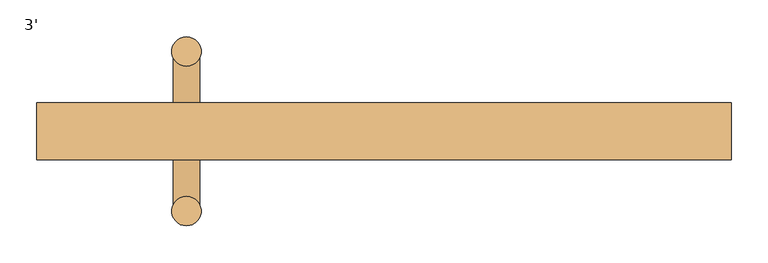
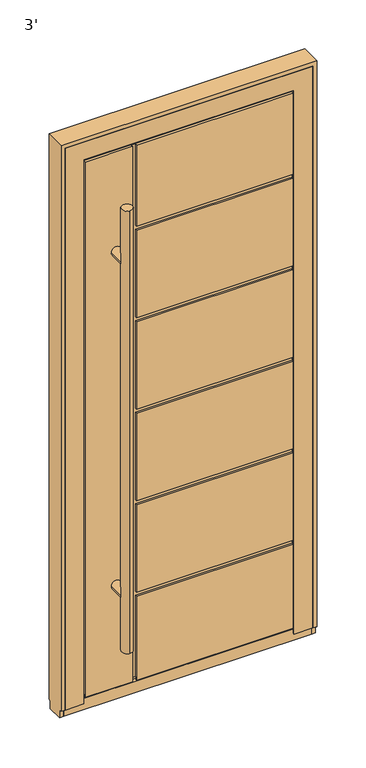
"""IFC4 building model written with IfcOpenShell, lengths in millimetres: door geometry, 3'."""

from ifc_helpers import new_model, si_unit, point, frame, frame_2d, origin, place, context, project, spatial, circle_curve, trimmed, segment, composite_curve, outline, extrude, faceted_brep, source, transform, mapped, element, save


def door_3_5c4206ef(model_context):
    return source(origin(), model_context, "Body", "SolidModel", [
        extrude(outline(composite_curve([segment(trimmed(circle_curve(frame_2d((-268.65, -90.8003001)), 20.0), [point((-268.65, -70.8003001))], [point((-268.65, -110.8003001))], False, "CARTESIAN"), True, "CONTINUOUS"), segment(trimmed(circle_curve(frame_2d((-268.65, -90.8003001)), 20.0), [point((-268.65, -110.8003001))], [point((-268.65, -70.8003001))], False, "CARTESIAN"), True, "CONTINUOUS")], self_intersect=False)), frame((0.0, 0.0, 210.0000003), z_axis=(0.0, 0.0, 1.0), x_axis=(1.0, 0.0, 0.0)), (0.0, 0.0, 1.0), 1724.5),
        extrude(outline(composite_curve([segment(trimmed(circle_curve(frame_2d((-268.65, 126.2003001)), 20.0), [point((-268.65, 146.2003001))], [point((-268.65, 106.2003001))], False, "CARTESIAN"), True, "CONTINUOUS"), segment(trimmed(circle_curve(frame_2d((-268.65, 126.2003001)), 20.0), [point((-268.65, 106.2003001))], [point((-268.65, 146.2003001))], False, "CARTESIAN"), True, "CONTINUOUS")], self_intersect=False)), frame((0.0, 0.0, 210.0000003), z_axis=(0.0, 0.0, 1.0), x_axis=(1.0, 0.0, 0.0)), (0.0, 0.0, 1.0), 1724.5),
        extrude(outline(composite_curve([segment(trimmed(circle_curve(frame_2d((422.2500003, -268.65)), 18.0), [point((422.2500003, -286.65))], [point((422.2500003, -250.65))], False, "CARTESIAN"), True, "CONTINUOUS"), segment(trimmed(circle_curve(frame_2d((422.2500003, -268.65)), 18.0), [point((422.2500003, -250.65))], [point((422.2500003, -286.65))], False, "CARTESIAN"), True, "CONTINUOUS")], self_intersect=False)), frame((0.0, -90.8, 0.0), z_axis=(0.0, 1.0, 0.0), x_axis=(0.0, 0.0, 1.0)), (0.0, 0.0, 1.0), 217.0),
        extrude(outline(composite_curve([segment(trimmed(circle_curve(frame_2d((1722.2500003, -268.65)), 18.0), [point((1722.2500003, -286.65))], [point((1722.2500003, -250.65))], False, "CARTESIAN"), True, "CONTINUOUS"), segment(trimmed(circle_curve(frame_2d((1722.2500003, -268.65)), 18.0), [point((1722.2500003, -250.65))], [point((1722.2500003, -286.65))], False, "CARTESIAN"), True, "CONTINUOUS")], self_intersect=False)), frame((0.0, -90.8, 0.0), z_axis=(0.0, 1.0, 0.0), x_axis=(0.0, 0.0, 1.0)), (0.0, 0.0, 1.0), 217.0),
        faceted_brep([(-193.65, -13.8, 366.5833337), (-193.65, -13.8, 708.166667), (383.65, -13.8, 708.166667), (383.65, -13.8, 723.166667), (-193.65, -13.8, 723.166667), (-193.65, -13.8, 1064.7500004), (383.65, -13.8, 1064.7500004), (383.65, -13.8, 1079.7500004), (-193.65, -13.8, 1079.7500004), (-193.65, -13.8, 1421.3333337), (383.65, -13.8, 1421.3333337), (383.65, -13.8, 1436.3333337), (-193.65, -13.8, 1436.3333337), (-193.65, -13.8, 1777.916667), (383.65, -13.8, 1777.916667), (383.65, -13.8, 1792.916667), (-193.65, -13.8, 1792.916667), (-193.65, -13.8, 2109.5000003), (-208.65, -13.8, 2109.5000003), (-208.65, -13.8, 35.0), (-193.65, -13.8, 35.0), (-193.65, -13.8, 351.5833337), (383.65, -13.8, 351.5833337), (383.65, -13.8, 366.5833337), (-193.65, -20.8, 366.5833337), (-193.65, -20.8, 708.166667), (383.65, -20.8, 708.166667), (383.65, -11.7997698, 2109.5000003), (383.65, -20.8, 2109.5000003), (383.65, -20.8, 1792.916667), (383.65, -20.8, 1777.916667), (383.65, -20.8, 1436.3333337), (383.65, -20.8, 1421.3333337), (383.65, -20.8, 1079.7500004), (383.65, -20.8, 1064.7500004), (383.65, -20.8, 723.166667), (383.65, -20.8, 366.5833337), (383.65, -20.8, 351.5833337), (383.65, -20.8, 24.0), (383.65, -18.8020472, 24.0), (383.65, -18.8020472, 35.0), (383.65, -11.7997698, 35.0), (-193.65, -20.8, 723.166667), (-193.65, -20.8, 1064.7500004), (-193.65, -20.8, 1079.7500004), (-193.65, -20.8, 1421.3333337), (-208.65, -20.8, 2109.5000003), (-208.65, -20.8, 24.0), (-208.65, -18.8020472, 24.0), (-208.65, -18.8020472, 35.0), (-193.65, -18.8020472, 35.0), (-383.65, -18.8020472, 35.0), (-383.65, -11.7997698, 35.0), (-193.65, -20.8, 351.5833337), (-193.65, -18.8020472, 24.0), (-193.65, -20.8, 24.0), (-383.65, -18.8020472, 24.0), (-383.65, -20.8, 24.0), (-383.65, -20.8, 2109.5000003), (-193.65, -20.8, 1777.916667), (-193.65, -20.8, 1436.3333337), (-193.65, -20.8, 2109.5000003), (-193.65, -20.8, 1792.916667), (408.65, 56.2, 10.0000003), (408.65, 53.2, 10.0000003), (-193.65, 53.2, 10.0000003), (-193.65, 56.2, 10.0000003), (-408.65, 53.2, 10.0000003), (-408.65, 56.2, 10.0000003), (-208.65, 56.2, 10.0000003), (-208.65, 53.2, 10.0000003), (408.65, 56.2, 351.5833337), (408.65, 53.2, 351.5833337), (408.65, 56.2, 366.5833337), (408.65, 56.2, 708.166667), (408.65, 53.2, 708.166667), (408.65, 53.2, 366.5833337), (408.65, 56.2, 1079.7500004), (408.65, 56.2, 1421.3333337), (408.65, 53.2, 1421.3333337), (408.65, 53.2, 1079.7500004), (408.65, 56.2, 723.166667), (408.65, 56.2, 1064.7500004), (408.65, 53.2, 1064.7500004), (408.65, 53.2, 723.166667), (408.65, 56.2, 1436.3333337), (408.65, 56.2, 1777.916667), (408.65, 53.2, 1777.916667), (408.65, 53.2, 1436.3333337), (408.65, 56.2, 2134.5000003), (408.65, 53.2, 2134.5000003), (408.65, 53.2, 1792.916667), (408.65, 56.2, 1792.916667), (393.15, 53.2, 351.5833337), (393.15, 53.2, 25.5), (-193.65, 53.2, 25.5), (393.15, 53.2, 708.166667), (393.15, 53.2, 366.5833337), (393.15, 53.2, 1421.3333337), (393.15, 53.2, 1079.7500004), (393.15, 53.2, 1064.7500004), (393.15, 53.2, 723.166667), (393.15, 53.2, 1777.916667), (393.15, 53.2, 1436.3333337), (-193.65, 53.2, 2134.5000003), (-193.65, 53.2, 2119.0000003), (393.15, 53.2, 2119.0000003), (393.15, 53.2, 1792.916667), (-393.15, 53.2, 25.5), (-393.15, 53.2, 2119.0000003), (-208.65, 53.2, 2119.0000003), (-208.65, 53.2, 2134.5000003), (-408.65, 53.2, 2134.5000003), (-208.65, 53.2, 25.5), (-193.65, 49.2, 351.5833337), (-193.65, 56.2, 351.5833337), (-193.65, 49.2, 25.5), (-193.65, 56.2, 366.5833337), (-193.65, 56.2, 708.166667), (-193.65, 56.2, 1079.7500004), (-193.65, 56.2, 1421.3333337), (-193.65, 56.2, 723.166667), (-193.65, 56.2, 1064.7500004), (-193.65, 56.2, 1436.3333337), (-193.65, 56.2, 1777.916667), (-193.65, 56.2, 1792.916667), (-193.65, 56.2, 2134.5000003), (-408.65, 56.2, 2134.5000003), (-208.65, 56.2, 2134.5000003), (-208.65, 49.2, 2119.0000003), (-208.65, 49.2, 25.5), (-383.65, -11.7997698, 2109.5000003), (393.15, -11.7997698, 2119.0000003), (-393.15, -11.7997698, 2119.0000003), (-393.15, -11.7997698, 25.5), (393.15, -11.7997698, 25.5), (393.15, 49.2, 351.5833337), (393.15, 49.2, 366.5833337), (393.15, 49.2, 708.166667), (393.15, 49.2, 723.166667), (393.15, 49.2, 1064.7500004), (393.15, 49.2, 1079.7500004), (393.15, 49.2, 1421.3333337), (393.15, 49.2, 1436.3333337), (393.15, 49.2, 1777.916667), (393.15, 49.2, 1792.916667), (-193.65, 49.2, 1777.916667), (-193.65, 49.2, 1436.3333337), (-193.65, 49.2, 1421.3333337), (-193.65, 49.2, 1079.7500004), (-193.65, 49.2, 1064.7500004), (-193.65, 49.2, 723.166667), (-193.65, 49.2, 708.166667), (-193.65, 49.2, 366.5833337), (-193.65, 49.2, 2119.0000003), (-193.65, 49.2, 1792.916667)], [[[0, 1, 2, 3, 4, 5, 6, 7, 8, 9, 10, 11, 12, 13, 14, 15, 16, 17, 18, 19, 20, 21, 22, 23]], [[1, 0, 24, 25]], [[1, 25, 26, 2]], [[27, 28, 29, 15, 14, 30, 31, 11, 10, 32, 33, 7, 6, 34, 35, 3, 2, 26, 36, 23, 22, 37, 38, 39, 40, 41]], [[42, 4, 3, 35]], [[5, 4, 42, 43]], [[5, 43, 34, 6]], [[44, 8, 7, 33]], [[9, 8, 44, 45]], [[19, 18, 46, 47, 48, 49]], [[41, 40, 50, 20, 19, 49, 51, 52]], [[53, 21, 20, 50, 54, 55]], [[21, 53, 37, 22]], [[24, 0, 23, 36]], [[40, 39, 54, 50]], [[56, 51, 49, 48]], [[39, 38, 55, 54]], [[57, 56, 48, 47]], [[33, 32, 45, 44]], [[35, 34, 43, 42]], [[36, 26, 25, 24]], [[55, 38, 37, 53]], [[58, 57, 47, 46]], [[31, 30, 59, 60]], [[28, 61, 62, 29]], [[63, 64, 65, 66]], [[67, 68, 69, 70]], [[64, 63, 71, 72]], [[73, 74, 75, 76]], [[77, 78, 79, 80]], [[81, 82, 83, 84]], [[85, 86, 87, 88]], [[89, 90, 91, 92]], [[65, 64, 72, 93, 94, 95]], [[76, 75, 96, 97]], [[80, 79, 98, 99]], [[84, 83, 100, 101]], [[88, 87, 102, 103]], [[90, 104, 105, 106, 107, 91]], [[108, 109, 110, 111, 112, 67, 70, 113]], [[114, 115, 66, 65, 95, 116]], [[63, 66, 115, 71]], [[74, 73, 117, 118]], [[78, 77, 119, 120]], [[82, 81, 121, 122]], [[86, 85, 123, 124]], [[89, 92, 125, 126]], [[68, 127, 128, 69]], [[68, 67, 112, 127]], [[129, 130, 113, 70, 69, 128, 111, 110]], [[58, 131, 52, 51, 56, 57]], [[132, 133, 134, 135], [131, 27, 41, 52]], [[106, 132, 135, 94, 93, 136, 137, 97, 96, 138, 139, 101, 100, 140, 141, 99, 98, 142, 143, 103, 102, 144, 145, 107]], [[94, 135, 134, 108, 113, 130, 116, 95]], [[133, 109, 108, 134]], [[146, 147, 143, 142, 148, 149, 141, 140, 150, 151, 139, 138, 152, 153, 137, 136, 114, 116, 130, 129, 154, 155, 145, 144]], [[149, 148, 120, 119]], [[149, 119, 77, 80, 99, 141]], [[122, 150, 140, 100, 83, 82]], [[151, 150, 122, 121]], [[151, 121, 81, 84, 101, 139]], [[118, 152, 138, 96, 75, 74]], [[153, 152, 118, 117]], [[153, 117, 73, 76, 97, 137]], [[115, 114, 136, 93, 72, 71]], [[9, 45, 32, 10]], [[60, 12, 11, 31]], [[13, 12, 60, 59]], [[13, 59, 30, 14]], [[62, 16, 15, 29]], [[16, 62, 61, 17]], [[124, 146, 144, 102, 87, 86]], [[125, 155, 154, 105, 104, 126]], [[120, 148, 142, 98, 79, 78]], [[147, 123, 85, 88, 103, 143]], [[147, 146, 124, 123]], [[155, 125, 92, 91, 107, 145]], [[90, 89, 126, 104]], [[127, 112, 111, 128]], [[132, 106, 105, 154, 129, 110, 109, 133]], [[27, 131, 58, 46, 18, 17, 61, 28]]]),
        faceted_brep([(-457.2, 56.2, 0.0), (-412.7, 56.2, 0.0), (-412.7, 47.2, 0.0), (-457.2, 47.1997571, 0.0), (-403.2, -16.2999958, 0.0), (-387.7, -16.2999958, 0.0), (-387.7, -20.8, 0.0), (-457.2, -20.8, 0.0), (-457.2, -11.8, 0.0), (-403.2, -11.8, 0.0), (457.2, -20.8, 0.0), (387.7, -20.8, 0.0), (387.7, -16.2999958, 0.0), (403.2, -16.2999958, 0.0), (403.2, -11.8, 0.0), (457.2, -11.8, 0.0), (412.7, 47.2, 0.0), (412.7, 56.2, 0.0), (457.2, 56.2, 0.0), (457.2, 47.1997571, 0.0), (-457.2, -20.8, 2189.5), (-457.2, 56.2, 2189.5), (-457.2, 47.1997571, -30.0), (-457.2, -11.8, -30.0), (457.2, 56.2, 2189.5), (412.7, 56.2, 2145.0), (-412.7, 56.2, 2145.0), (457.2, -20.8, 2189.5), (457.2, -11.8, -30.0), (457.2, 47.1997571, -30.0), (-387.7, -20.8, 2120.0), (387.7, -20.8, 2120.0), (-403.2, 47.2, 2135.5), (-403.2, -16.2999958, 2135.5), (-403.2, -11.8, 14.5), (-403.2, 47.2, 14.5), (403.2, 47.2, 2135.5), (403.2, -16.2999958, 2135.5), (403.2, 47.2, 14.5), (403.2, -11.8, 14.5), (-412.7, 47.2, 2145.0), (412.7, 47.2, 2145.0), (387.7, -16.2999958, 2120.0), (-387.7, -16.2999958, 2120.0)], [[[0, 1, 2, 3]], [[4, 5, 6, 7, 8, 9]], [[10, 11, 12, 13, 14, 15]], [[16, 17, 18, 19]], [[7, 20, 21, 0, 3, 22, 23, 8]], [[1, 0, 21, 24, 18, 17, 25, 26]], [[21, 20, 27, 24]], [[18, 24, 27, 10, 15, 28, 29, 19]], [[7, 6, 30, 31, 11, 10, 27, 20]], [[32, 33, 4, 9, 34, 35]], [[33, 32, 36, 37]], [[37, 36, 38, 39, 14, 13]], [[40, 2, 1, 26]], [[16, 19, 29, 22, 3, 2, 40, 41], [36, 32, 35, 38]], [[5, 4, 33, 37, 13, 12, 42, 43]], [[6, 5, 43, 30]], [[26, 25, 41, 40]], [[31, 30, 43, 42]], [[17, 16, 41, 25]], [[12, 11, 31, 42]], [[23, 28, 15, 14, 39, 34, 9, 8]], [[38, 35, 34, 39]], [[23, 22, 29, 28]]]),
        faceted_brep([(-457.2, 47.2, -30.0), (-457.2, -11.8, -30.0), (-472.2, -11.8, -30.0), (-472.2, 47.2, -30.0), (-457.2, 56.2, 2189.5), (-457.2, -20.8, 2189.5), (-457.2, -20.8, 0.0), (-457.2, -11.8, 0.0), (-457.2, 47.2, 0.0), (-457.2, 56.2, 0.0), (472.2, -11.8, 0.0), (457.2, -11.8, 0.0), (457.2, -11.8, -30.0), (472.2, -11.8, -30.0), (-472.2, -11.8, 0.0), (-472.2, -20.8, 2204.5), (-472.2, 56.2, 2204.5), (-472.2, 56.2, 0.0), (-472.2, 47.2, 0.0), (-472.2, -20.8, 0.0), (457.2, 47.2, 0.0), (472.2, 47.2, 0.0), (472.2, 47.2, -30.0), (457.2, 47.2, -30.0), (457.2, -20.8, 2189.5), (457.2, 56.2, 2189.5), (457.2, 56.2, 0.0), (457.2, -20.8, 0.0), (472.2, 56.2, 2204.5), (472.2, 56.2, 0.0), (472.2, -20.8, 0.0), (472.2, -20.8, 2204.5)], [[[0, 1, 2, 3]], [[4, 5, 6, 7, 1, 0, 8, 9]], [[10, 11, 12, 13]], [[7, 14, 2, 1]], [[15, 16, 17, 18, 3, 2, 14, 19]], [[20, 21, 22, 23]], [[18, 8, 0, 3]], [[24, 25, 26, 20, 23, 12, 11, 27]], [[25, 4, 9, 17, 16, 28, 29, 26]], [[21, 20, 26, 29]], [[8, 18, 17, 9]], [[22, 13, 12, 23]], [[11, 10, 30, 27]], [[14, 7, 6, 19]], [[5, 24, 27, 30, 31, 15, 19, 6]], [[28, 31, 30, 10, 13, 22, 21, 29]], [[5, 4, 25, 24]], [[16, 15, 31, 28]]]),
    ])


if __name__ == "__main__":
    model = new_model("IFC4")
    model_context = context("Model", 3, world=origin())
    ifc_project = project(units=[si_unit("LENGTHUNIT", "METRE", prefix="MILLI")], contexts=[model_context])
    site = spatial("IfcSite", under=ifc_project)
    building = spatial("IfcBuilding", under=site)
    placement = place(None, origin())
    door_3_shape = door_3_5c4206ef(model_context)
    element("IfcDoor", 1, ObjectType="3'", at=placement, inside=building, context=model_context, shape_type="MappedRepresentation", body=[
        mapped(door_3_shape, transform((0.0, 0.0, 0.0), x_axis=(1.0, 0.0, 0.0), y_axis=(0.0, 1.0, 0.0), z_axis=(0.0, 0.0, 1.0))),
    ])
    save(model, "model.ifc")

# Revit data of these elements
# Type "3'"
#   Type Mark = "15"
#   Water resistance = "up to Class E900, EN 12208:2001"
#   Uniclass2015Version = "v1.21"
#   Uniclass2015Reference = "Ss_25_30_20_30"
#   Uniclass2015Description = "Frame and door leaf system"
#   URL = "www.aluprof.com"
#   Type IFC Predefined Type = "USERDEFINED"
#   Right-hand / Left-hand door [instance default] = ""
#   Resistance to wind load = "up to Class C5/B5, EN 12210:2001"
#   Insert type = "ST"
#   Hardware [instance default] = ""
#   Product page = "https://aluprof.com/en/architects/offer/window-and-door-systems/panel-doors#visualisation"
#   Operation = "SinglePanelOutwardOpening"
#   Opening type = "Outward"
#   NBSReference = "25-50-20/125"
#   NBSDescription = "Frame and door leaf system"
#   Important = "The actual acceptable construction dimensions are dependent on the selection of profiles and hardware, glazing type, construction weight and the construction’s operating conditions. These should be determined by a suitably qualified person, and using ALUPROF’s calculation software"
#   IfcExportType = "USERDEFINED"
#   IfcExportAs = "IfcDoorType"
#   Handle type [instance default] = ""
#   Manufacturer = "ALUPROF SA"
#   Export Type to IFC As = "IfcDoorType"
#   Door sill type [instance default] = ""
#   Description = "External single-leaf panel door outward opening"
#   Model = "MB-86 ST Panel Door AD07"
#   Content of the recyclate in the material = "69.2%"
#   COBie.Type.WarrantyDurationParts = ""
#   COBie.Type.Name = ""
#   COBie.Type.Manufacturer = "ALUPROF SA"
#   COBie.Space.Name = ""
#   COBie.Floor.Name = ""
#   COBie.Facility.Name = ""
#   COBie.CreatedOn = ""
#   COBie.Component.WarrantyStartDate = ""
#   COBie.Component.Name = "MB-86 ST Panel Door AD07"
#   Burglar resistance = "RC2"
#   Air permeability = "up to Class 4, EN 12207:2001"
#   Width of the active leaf = 2' - 8.17717"
#   Placement in wall = 0' - 0.7874"
#   Thickness = 0' - 3.0315"
#   Height of the opening sash = 6' - 11.64173"
#   Handle Offset = 3' - 5.33858"
#   Rough Height = 7' - 4.61024"
#   Rough Width = 3' - 1.1811"
#   Height = 7' - 2.20079"
#   Width = 3' - 0"
#   Construction depth = 0' - 3.0315"
#   Clear opening width = 2' - 3.94882"
#   Clear opening height = 6' - 10.67717"
#   Height of the array = 1' - 1.44816"
#   Schedule No. [instance default] = 1
#   Handrail [instance default] = yes
#   IsExternal = yes
#   Handle [instance default] = no
#   Door closer [instance default] = no
#   Function = 1
#   COBie.Type = yes
#   COBie = yes
#   Access control [instance default] = no
#   Panel = element 387710
#   Wall Closure = (empty or 0)
